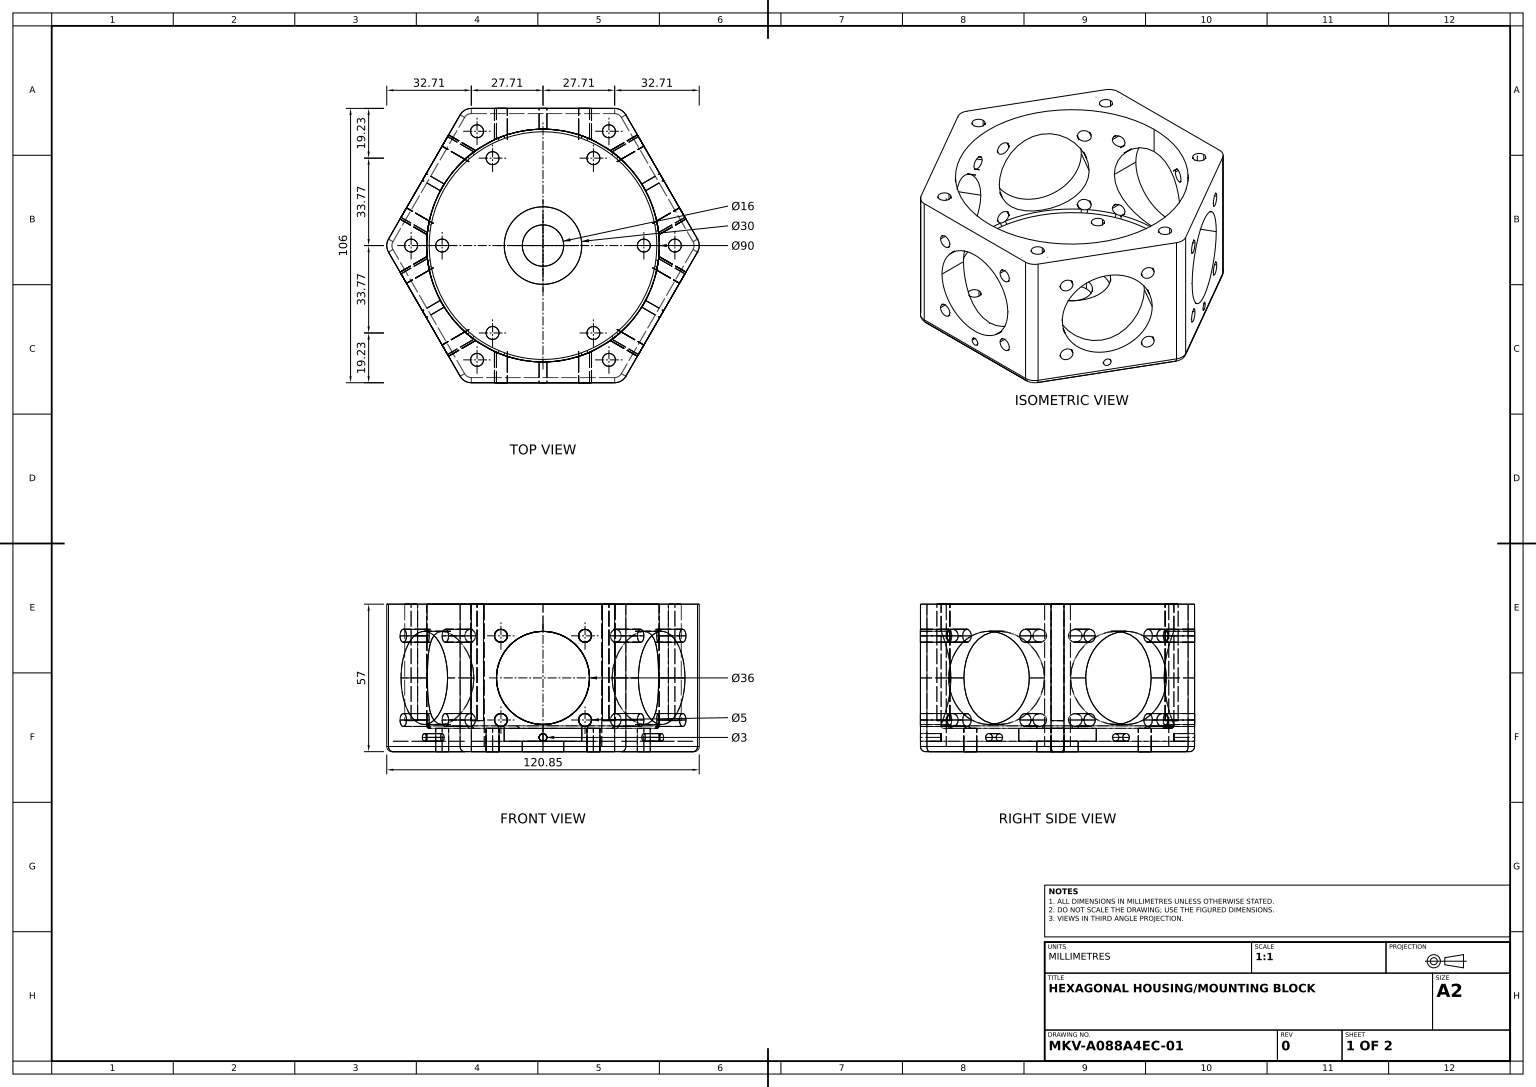
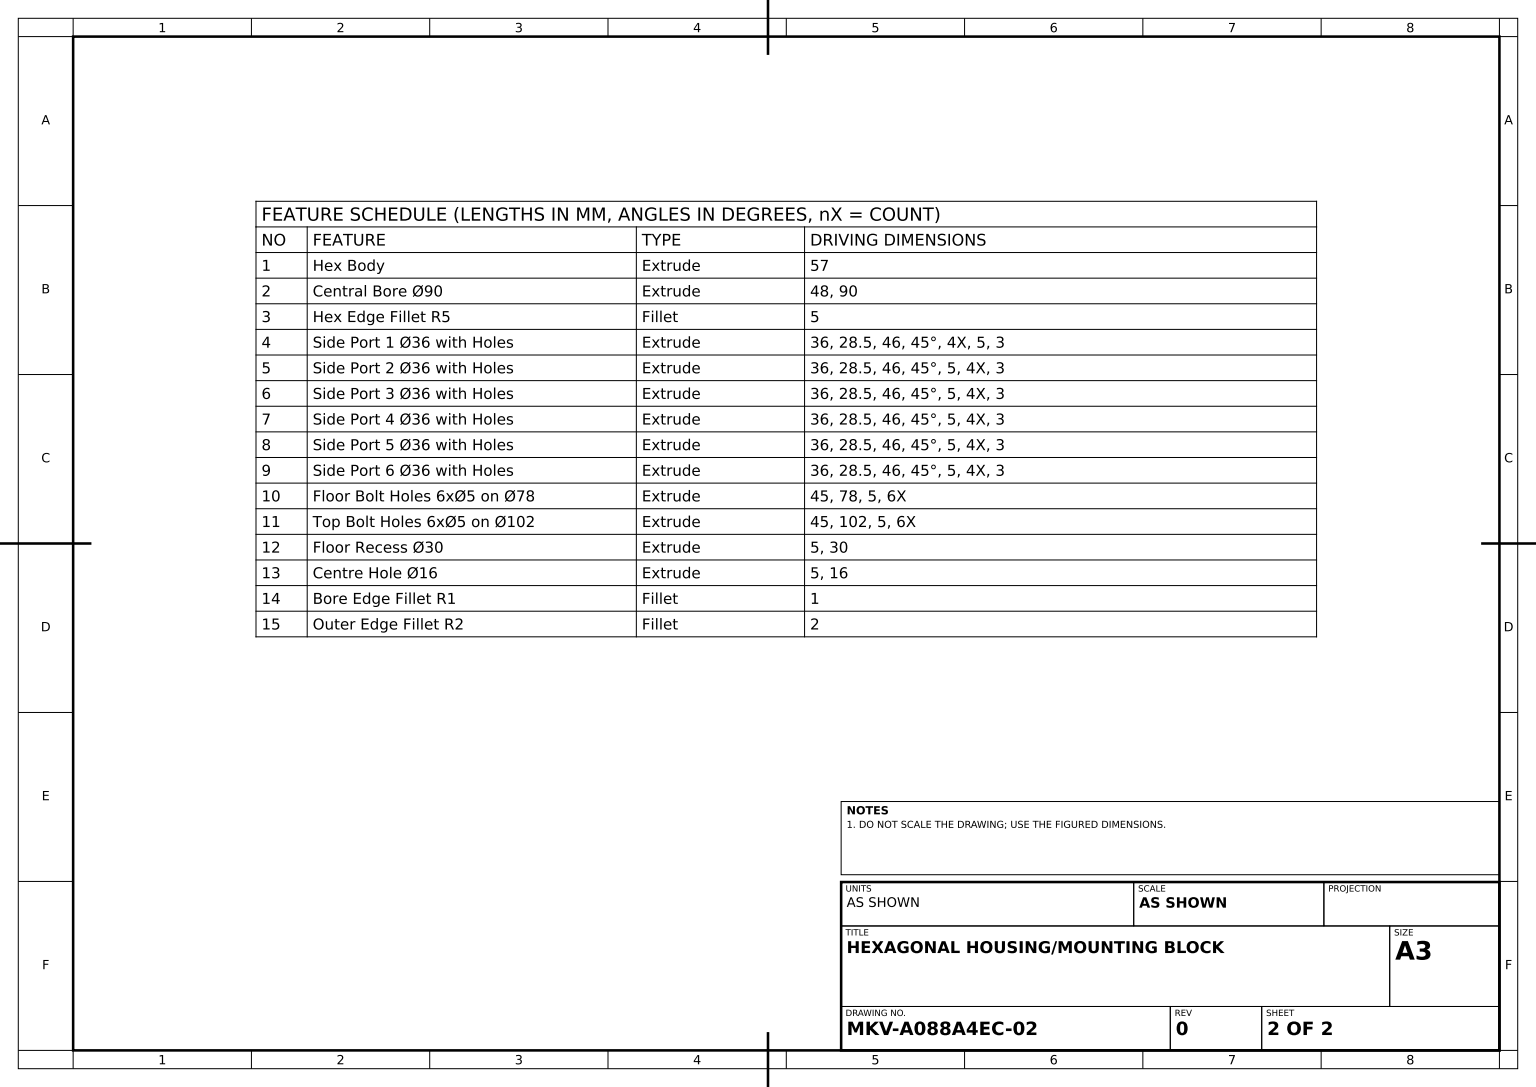
from build123d import *

# Parameters (mm, degrees)
HEX_BODY_DEPTH                       = 57
CENTRAL_BORE_SKETCH_R                = 45
CENTRAL_BORE_90_DEPTH                = 48
HEX_EDGE_FILLET_R5_R                 = 5
SIDE_PORT_1_36_WITH_HOLES_REACH      = 136.671
SIDE_PORT_1_36_WITH_HOLES_END_RADIUS = 45
SIDE_PORT_1_SKETCH_R                 = 18
SIDE_PORT_1_SKETCH_R_2               = 2.5
SIDE_PORT_1_SKETCH_R_3               = 1.5
SIDE_PORT_2_36_WITH_HOLES_REACH      = 146.479
SIDE_PORT_2_36_WITH_HOLES_END_RADIUS = 45
SIDE_PORT_2_SKETCH_R                 = 18
SIDE_PORT_2_SKETCH_R_2               = 2.5
SIDE_PORT_2_SKETCH_R_3               = 1.5
SIDE_PORT_3_36_WITH_HOLES_REACH      = 146.479
SIDE_PORT_3_36_WITH_HOLES_END_RADIUS = 45
SIDE_PORT_3_SKETCH_R                 = 18
SIDE_PORT_3_SKETCH_R_2               = 2.5
SIDE_PORT_3_SKETCH_R_3               = 1.5
SIDE_PORT_4_36_WITH_HOLES_REACH      = 136.671
SIDE_PORT_4_36_WITH_HOLES_END_RADIUS = 45
SIDE_PORT_4_SKETCH_R                 = 18
SIDE_PORT_4_SKETCH_R_2               = 2.5
SIDE_PORT_4_SKETCH_R_3               = 1.5
SIDE_PORT_5_36_WITH_HOLES_REACH      = 146.479
SIDE_PORT_5_36_WITH_HOLES_END_RADIUS = 45
SIDE_PORT_5_SKETCH_R                 = 18
SIDE_PORT_5_SKETCH_R_2               = 2.5
SIDE_PORT_5_SKETCH_R_3               = 1.5
SIDE_PORT_6_36_WITH_HOLES_REACH      = 146.479
SIDE_PORT_6_36_WITH_HOLES_END_RADIUS = 45
SIDE_PORT_6_SKETCH_R                 = 18
SIDE_PORT_6_SKETCH_R_2               = 2.5
SIDE_PORT_6_SKETCH_R_3               = 1.5
FLOOR_BOLT_CIRCLE_SKETCH_R           = 2.5
FLOOR_BOLT_HOLES_6X_5_ON_78_DEPTH    = 45
TOP_BOLT_CIRCLE_SKETCH_R             = 2.5
TOP_BOLT_HOLES_6X_5_ON_102_DEPTH     = 45
FLOOR_RECESS_SKETCH_R                = 15
FLOOR_RECESS_30_DEPTH                = 5
CENTRE_HOLE_SKETCH_R                 = 8
CENTRE_HOLE_16_DEPTH                 = 5
BORE_EDGE_FILLET_R1_R                = 1
OUTER_EDGE_FILLET_R2_R               = 2


with BuildPart() as part:
    # Hex Body Profile Sketch → Hex Body (new body)
    with BuildSketch(Plane(origin=(0, 0, 0), x_dir=(1, 0, 0), z_dir=(0, 1, 0))):
        Polygon((61.199128534, 0), (30.599564267, 53), (-30.599564267, 53), (-61.199128534, 0), (-30.599564267, -53), (30.599564267, -53), align=None)
    extrude(amount=HEX_BODY_DEPTH)

    # Central Bore Sketch → Central Bore Ø90 (cut)
    with BuildSketch(Plane(origin=(0, 57, 0), x_dir=(1, 0, 0), z_dir=(0, 1, 0))):
        with Locations(Location((0, 0, 0), (0, 0, 270))):
            Circle(CENTRAL_BORE_SKETCH_R)
    extrude(amount=-CENTRAL_BORE_90_DEPTH, mode=Mode.SUBTRACT)

    # Hex Edge Fillet R5
    hex_edge_fillet_r5_edges = [part.edges().sort_by_distance(p)[0] for p in [
        (30.599564267, 28.5, 53),
        (-30.599564267, 28.5, 53),
        (-61.199128534, 28.5, 0),
        (-30.599564267, 28.5, -53),
        (30.599564267, 28.5, -53),
        (61.199128534, 28.5, 0),
    ]]
    fillet(hex_edge_fillet_r5_edges, radius=HEX_EDGE_FILLET_R5_R)

    # Side Port 1 Ø36 with Holes: up to this cylinder (the profile starts outside it)
    side_port_1_36_with_holes_end = Plane(origin=(0, 25.131728, 0), z_dir=(0, 1, 0)) * Cylinder(SIDE_PORT_1_36_WITH_HOLES_END_RADIUS, 403.605456, mode=Mode.PRIVATE)
    # Side Port 1 Sketch → Side Port 1 Ø36 with Holes (cut, up to the surface)
    with BuildSketch(Plane(origin=(0, 0, -53), x_dir=(-1, 0, 0), z_dir=(0, 0, -1)), mode=Mode.PRIVATE) as side_port_1_36_with_holes_sk1:
        with Locations((0, 28.5)):
            Circle(SIDE_PORT_1_SKETCH_R)
    side_port_1_36_with_holes_tool1 = extrude(side_port_1_36_with_holes_sk1.sketch, amount=-SIDE_PORT_1_36_WITH_HOLES_REACH, mode=Mode.PRIVATE) - side_port_1_36_with_holes_end
    add(side_port_1_36_with_holes_tool1.solids().sort_by_distance((0, 28.5, -53))[0], mode=Mode.SUBTRACT)
    # Side Port 1 Sketch → Side Port 1 Ø36 with Holes (cut, up to the surface)
    with BuildSketch(Plane(origin=(0, 0, -53), x_dir=(-1, 0, 0), z_dir=(0, 0, -1)), mode=Mode.PRIVATE) as side_port_1_36_with_holes_sk2:
        with Locations((16.263455967, 44.763455967)):
            Circle(SIDE_PORT_1_SKETCH_R_2)
    side_port_1_36_with_holes_tool2 = extrude(side_port_1_36_with_holes_sk2.sketch, amount=-SIDE_PORT_1_36_WITH_HOLES_REACH, mode=Mode.PRIVATE) - side_port_1_36_with_holes_end
    add(side_port_1_36_with_holes_tool2.solids().sort_by_distance((-16.263456, 44.763456, -53))[0], mode=Mode.SUBTRACT)
    # Side Port 1 Sketch → Side Port 1 Ø36 with Holes (cut, up to the surface)
    with BuildSketch(Plane(origin=(0, 0, -53), x_dir=(-1, 0, 0), z_dir=(0, 0, -1)), mode=Mode.PRIVATE) as side_port_1_36_with_holes_sk3:
        with Locations((16.263455967, 12.236544033)):
            Circle(SIDE_PORT_1_SKETCH_R_2)
    side_port_1_36_with_holes_tool3 = extrude(side_port_1_36_with_holes_sk3.sketch, amount=-SIDE_PORT_1_36_WITH_HOLES_REACH, mode=Mode.PRIVATE) - side_port_1_36_with_holes_end
    add(side_port_1_36_with_holes_tool3.solids().sort_by_distance((-16.263456, 12.236544, -53))[0], mode=Mode.SUBTRACT)
    # Side Port 1 Sketch → Side Port 1 Ø36 with Holes (cut, up to the surface)
    with BuildSketch(Plane(origin=(0, 0, -53), x_dir=(-1, 0, 0), z_dir=(0, 0, -1)), mode=Mode.PRIVATE) as side_port_1_36_with_holes_sk4:
        with Locations((-16.263455967, 12.236544033)):
            Circle(SIDE_PORT_1_SKETCH_R_2)
    side_port_1_36_with_holes_tool4 = extrude(side_port_1_36_with_holes_sk4.sketch, amount=-SIDE_PORT_1_36_WITH_HOLES_REACH, mode=Mode.PRIVATE) - side_port_1_36_with_holes_end
    add(side_port_1_36_with_holes_tool4.solids().sort_by_distance((16.263456, 12.236544, -53))[0], mode=Mode.SUBTRACT)
    # Side Port 1 Sketch → Side Port 1 Ø36 with Holes (cut, up to the surface)
    with BuildSketch(Plane(origin=(0, 0, -53), x_dir=(-1, 0, 0), z_dir=(0, 0, -1)), mode=Mode.PRIVATE) as side_port_1_36_with_holes_sk5:
        with Locations((-16.263455967, 44.763455967)):
            Circle(SIDE_PORT_1_SKETCH_R_2)
    side_port_1_36_with_holes_tool5 = extrude(side_port_1_36_with_holes_sk5.sketch, amount=-SIDE_PORT_1_36_WITH_HOLES_REACH, mode=Mode.PRIVATE) - side_port_1_36_with_holes_end
    add(side_port_1_36_with_holes_tool5.solids().sort_by_distance((16.263456, 44.763456, -53))[0], mode=Mode.SUBTRACT)
    # Side Port 1 Sketch → Side Port 1 Ø36 with Holes (cut, up to the surface)
    with BuildSketch(Plane(origin=(0, 0, -53), x_dir=(-1, 0, 0), z_dir=(0, 0, -1)), mode=Mode.PRIVATE) as side_port_1_36_with_holes_sk6:
        with Locations((0, 5.5)):
            Circle(SIDE_PORT_1_SKETCH_R_3)
    side_port_1_36_with_holes_tool6 = extrude(side_port_1_36_with_holes_sk6.sketch, amount=-SIDE_PORT_1_36_WITH_HOLES_REACH, mode=Mode.PRIVATE) - side_port_1_36_with_holes_end
    add(side_port_1_36_with_holes_tool6.solids().sort_by_distance((0, 5.5, -53))[0], mode=Mode.SUBTRACT)

    # Side Port 2 Ø36 with Holes: up to this cylinder (the profile starts outside it)
    side_port_2_36_with_holes_end = Plane(origin=(0, 25.131728, 0), z_dir=(0, 1, 0)) * Cylinder(SIDE_PORT_2_36_WITH_HOLES_END_RADIUS, 423.221456, mode=Mode.PRIVATE)
    # Side Port 2 Sketch → Side Port 2 Ø36 with Holes (cut, up to the surface)
    with BuildSketch(Plane(origin=(-45.899346401, 0, -26.5), x_dir=(-0.49999999999999484, 0, 0.8660254037844416), z_dir=(-0.8660254037844416, 0, -0.49999999999999484)), mode=Mode.PRIVATE) as side_port_2_36_with_holes_sk1:
        with Locations((0, 28.5)):
            Circle(SIDE_PORT_2_SKETCH_R)
    side_port_2_36_with_holes_tool1 = extrude(side_port_2_36_with_holes_sk1.sketch, amount=-SIDE_PORT_2_36_WITH_HOLES_REACH, mode=Mode.PRIVATE) - side_port_2_36_with_holes_end
    add(side_port_2_36_with_holes_tool1.solids().sort_by_distance((-45.899346, 28.5, -26.5))[0], mode=Mode.SUBTRACT)
    # Side Port 2 Sketch → Side Port 2 Ø36 with Holes (cut, up to the surface)
    with BuildSketch(Plane(origin=(-45.899346401, 0, -26.5), x_dir=(-0.49999999999999484, 0, 0.8660254037844416), z_dir=(-0.8660254037844416, 0, -0.49999999999999484)), mode=Mode.PRIVATE) as side_port_2_36_with_holes_sk2:
        with Locations((16.263455967, 44.763455967)):
            Circle(SIDE_PORT_2_SKETCH_R_2)
    side_port_2_36_with_holes_tool2 = extrude(side_port_2_36_with_holes_sk2.sketch, amount=-SIDE_PORT_2_36_WITH_HOLES_REACH, mode=Mode.PRIVATE) - side_port_2_36_with_holes_end
    add(side_port_2_36_with_holes_tool2.solids().sort_by_distance((-54.031074, 44.763456, -12.415434))[0], mode=Mode.SUBTRACT)
    # Side Port 2 Sketch → Side Port 2 Ø36 with Holes (cut, up to the surface)
    with BuildSketch(Plane(origin=(-45.899346401, 0, -26.5), x_dir=(-0.49999999999999484, 0, 0.8660254037844416), z_dir=(-0.8660254037844416, 0, -0.49999999999999484)), mode=Mode.PRIVATE) as side_port_2_36_with_holes_sk3:
        with Locations((16.263455967, 12.236544033)):
            Circle(SIDE_PORT_2_SKETCH_R_2)
    side_port_2_36_with_holes_tool3 = extrude(side_port_2_36_with_holes_sk3.sketch, amount=-SIDE_PORT_2_36_WITH_HOLES_REACH, mode=Mode.PRIVATE) - side_port_2_36_with_holes_end
    add(side_port_2_36_with_holes_tool3.solids().sort_by_distance((-54.031074, 12.236544, -12.415434))[0], mode=Mode.SUBTRACT)
    # Side Port 2 Sketch → Side Port 2 Ø36 with Holes (cut, up to the surface)
    with BuildSketch(Plane(origin=(-45.899346401, 0, -26.5), x_dir=(-0.49999999999999484, 0, 0.8660254037844416), z_dir=(-0.8660254037844416, 0, -0.49999999999999484)), mode=Mode.PRIVATE) as side_port_2_36_with_holes_sk4:
        with Locations((-16.263455967, 12.236544033)):
            Circle(SIDE_PORT_2_SKETCH_R_2)
    side_port_2_36_with_holes_tool4 = extrude(side_port_2_36_with_holes_sk4.sketch, amount=-SIDE_PORT_2_36_WITH_HOLES_REACH, mode=Mode.PRIVATE) - side_port_2_36_with_holes_end
    add(side_port_2_36_with_holes_tool4.solids().sort_by_distance((-37.767618, 12.236544, -40.584566))[0], mode=Mode.SUBTRACT)
    # Side Port 2 Sketch → Side Port 2 Ø36 with Holes (cut, up to the surface)
    with BuildSketch(Plane(origin=(-45.899346401, 0, -26.5), x_dir=(-0.49999999999999484, 0, 0.8660254037844416), z_dir=(-0.8660254037844416, 0, -0.49999999999999484)), mode=Mode.PRIVATE) as side_port_2_36_with_holes_sk5:
        with Locations((-16.263455967, 44.763455967)):
            Circle(SIDE_PORT_2_SKETCH_R_2)
    side_port_2_36_with_holes_tool5 = extrude(side_port_2_36_with_holes_sk5.sketch, amount=-SIDE_PORT_2_36_WITH_HOLES_REACH, mode=Mode.PRIVATE) - side_port_2_36_with_holes_end
    add(side_port_2_36_with_holes_tool5.solids().sort_by_distance((-37.767618, 44.763456, -40.584566))[0], mode=Mode.SUBTRACT)
    # Side Port 2 Sketch → Side Port 2 Ø36 with Holes (cut, up to the surface)
    with BuildSketch(Plane(origin=(-45.899346401, 0, -26.5), x_dir=(-0.49999999999999484, 0, 0.8660254037844416), z_dir=(-0.8660254037844416, 0, -0.49999999999999484)), mode=Mode.PRIVATE) as side_port_2_36_with_holes_sk6:
        with Locations((0, 5.5)):
            Circle(SIDE_PORT_2_SKETCH_R_3)
    side_port_2_36_with_holes_tool6 = extrude(side_port_2_36_with_holes_sk6.sketch, amount=-SIDE_PORT_2_36_WITH_HOLES_REACH, mode=Mode.PRIVATE) - side_port_2_36_with_holes_end
    add(side_port_2_36_with_holes_tool6.solids().sort_by_distance((-45.899346, 5.5, -26.5))[0], mode=Mode.SUBTRACT)

    # Side Port 3 Ø36 with Holes: up to this cylinder (the profile starts outside it)
    side_port_3_36_with_holes_end = Plane(origin=(0, 25.131728, 0), z_dir=(0, 1, 0)) * Cylinder(SIDE_PORT_3_36_WITH_HOLES_END_RADIUS, 423.221456, mode=Mode.PRIVATE)
    # Side Port 3 Sketch → Side Port 3 Ø36 with Holes (cut, up to the surface)
    with BuildSketch(Plane(origin=(-45.899346401, 0, 26.5), x_dir=(0.5000000000000071, 0, 0.8660254037844346), z_dir=(-0.8660254037844345, 0, 0.500000000000007)), mode=Mode.PRIVATE) as side_port_3_36_with_holes_sk1:
        with Locations((0, 28.5)):
            Circle(SIDE_PORT_3_SKETCH_R)
    side_port_3_36_with_holes_tool1 = extrude(side_port_3_36_with_holes_sk1.sketch, amount=-SIDE_PORT_3_36_WITH_HOLES_REACH, mode=Mode.PRIVATE) - side_port_3_36_with_holes_end
    add(side_port_3_36_with_holes_tool1.solids().sort_by_distance((-45.899346, 28.5, 26.5))[0], mode=Mode.SUBTRACT)
    # Side Port 3 Sketch → Side Port 3 Ø36 with Holes (cut, up to the surface)
    with BuildSketch(Plane(origin=(-45.899346401, 0, 26.5), x_dir=(0.5000000000000071, 0, 0.8660254037844346), z_dir=(-0.8660254037844345, 0, 0.500000000000007)), mode=Mode.PRIVATE) as side_port_3_36_with_holes_sk2:
        with Locations((16.263455967, 44.763455967)):
            Circle(SIDE_PORT_3_SKETCH_R_2)
    side_port_3_36_with_holes_tool2 = extrude(side_port_3_36_with_holes_sk2.sketch, amount=-SIDE_PORT_3_36_WITH_HOLES_REACH, mode=Mode.PRIVATE) - side_port_3_36_with_holes_end
    add(side_port_3_36_with_holes_tool2.solids().sort_by_distance((-37.767618, 44.763456, 40.584566))[0], mode=Mode.SUBTRACT)
    # Side Port 3 Sketch → Side Port 3 Ø36 with Holes (cut, up to the surface)
    with BuildSketch(Plane(origin=(-45.899346401, 0, 26.5), x_dir=(0.5000000000000071, 0, 0.8660254037844346), z_dir=(-0.8660254037844345, 0, 0.500000000000007)), mode=Mode.PRIVATE) as side_port_3_36_with_holes_sk3:
        with Locations((16.263455967, 12.236544033)):
            Circle(SIDE_PORT_3_SKETCH_R_2)
    side_port_3_36_with_holes_tool3 = extrude(side_port_3_36_with_holes_sk3.sketch, amount=-SIDE_PORT_3_36_WITH_HOLES_REACH, mode=Mode.PRIVATE) - side_port_3_36_with_holes_end
    add(side_port_3_36_with_holes_tool3.solids().sort_by_distance((-37.767618, 12.236544, 40.584566))[0], mode=Mode.SUBTRACT)
    # Side Port 3 Sketch → Side Port 3 Ø36 with Holes (cut, up to the surface)
    with BuildSketch(Plane(origin=(-45.899346401, 0, 26.5), x_dir=(0.5000000000000071, 0, 0.8660254037844346), z_dir=(-0.8660254037844345, 0, 0.500000000000007)), mode=Mode.PRIVATE) as side_port_3_36_with_holes_sk4:
        with Locations((-16.263455967, 12.236544033)):
            Circle(SIDE_PORT_3_SKETCH_R_2)
    side_port_3_36_with_holes_tool4 = extrude(side_port_3_36_with_holes_sk4.sketch, amount=-SIDE_PORT_3_36_WITH_HOLES_REACH, mode=Mode.PRIVATE) - side_port_3_36_with_holes_end
    add(side_port_3_36_with_holes_tool4.solids().sort_by_distance((-54.031074, 12.236544, 12.415434))[0], mode=Mode.SUBTRACT)
    # Side Port 3 Sketch → Side Port 3 Ø36 with Holes (cut, up to the surface)
    with BuildSketch(Plane(origin=(-45.899346401, 0, 26.5), x_dir=(0.5000000000000071, 0, 0.8660254037844346), z_dir=(-0.8660254037844345, 0, 0.500000000000007)), mode=Mode.PRIVATE) as side_port_3_36_with_holes_sk5:
        with Locations((-16.263455967, 44.763455967)):
            Circle(SIDE_PORT_3_SKETCH_R_2)
    side_port_3_36_with_holes_tool5 = extrude(side_port_3_36_with_holes_sk5.sketch, amount=-SIDE_PORT_3_36_WITH_HOLES_REACH, mode=Mode.PRIVATE) - side_port_3_36_with_holes_end
    add(side_port_3_36_with_holes_tool5.solids().sort_by_distance((-54.031074, 44.763456, 12.415434))[0], mode=Mode.SUBTRACT)
    # Side Port 3 Sketch → Side Port 3 Ø36 with Holes (cut, up to the surface)
    with BuildSketch(Plane(origin=(-45.899346401, 0, 26.5), x_dir=(0.5000000000000071, 0, 0.8660254037844346), z_dir=(-0.8660254037844345, 0, 0.500000000000007)), mode=Mode.PRIVATE) as side_port_3_36_with_holes_sk6:
        with Locations((0, 5.5)):
            Circle(SIDE_PORT_3_SKETCH_R_3)
    side_port_3_36_with_holes_tool6 = extrude(side_port_3_36_with_holes_sk6.sketch, amount=-SIDE_PORT_3_36_WITH_HOLES_REACH, mode=Mode.PRIVATE) - side_port_3_36_with_holes_end
    add(side_port_3_36_with_holes_tool6.solids().sort_by_distance((-45.899346, 5.5, 26.5))[0], mode=Mode.SUBTRACT)

    # Side Port 4 Ø36 with Holes: up to this cylinder (the profile starts outside it)
    side_port_4_36_with_holes_end = Plane(origin=(0, 25.131728, 0), z_dir=(0, 1, 0)) * Cylinder(SIDE_PORT_4_36_WITH_HOLES_END_RADIUS, 403.605456, mode=Mode.PRIVATE)
    # Side Port 4 Sketch → Side Port 4 Ø36 with Holes (cut, up to the surface)
    with BuildSketch(Plane.XY.offset(53), mode=Mode.PRIVATE) as side_port_4_36_with_holes_sk1:
        with Locations(Location((0, 28.5, 0), (0, 0, 180))):
            Circle(SIDE_PORT_4_SKETCH_R)
    side_port_4_36_with_holes_tool1 = extrude(side_port_4_36_with_holes_sk1.sketch, amount=-SIDE_PORT_4_36_WITH_HOLES_REACH, mode=Mode.PRIVATE) - side_port_4_36_with_holes_end
    add(side_port_4_36_with_holes_tool1.solids().sort_by_distance((0, 28.5, 53))[0], mode=Mode.SUBTRACT)
    # Side Port 4 Sketch → Side Port 4 Ø36 with Holes (cut, up to the surface)
    with BuildSketch(Plane.XY.offset(53), mode=Mode.PRIVATE) as side_port_4_36_with_holes_sk2:
        with Locations(Location((16.263455967, 44.763455967, 0), (0, 0, 180))):
            Circle(SIDE_PORT_4_SKETCH_R_2)
    side_port_4_36_with_holes_tool2 = extrude(side_port_4_36_with_holes_sk2.sketch, amount=-SIDE_PORT_4_36_WITH_HOLES_REACH, mode=Mode.PRIVATE) - side_port_4_36_with_holes_end
    add(side_port_4_36_with_holes_tool2.solids().sort_by_distance((16.263456, 44.763456, 53))[0], mode=Mode.SUBTRACT)
    # Side Port 4 Sketch → Side Port 4 Ø36 with Holes (cut, up to the surface)
    with BuildSketch(Plane.XY.offset(53), mode=Mode.PRIVATE) as side_port_4_36_with_holes_sk3:
        with Locations(Location((16.263455967, 12.236544033, 0), (0, 0, 180))):
            Circle(SIDE_PORT_4_SKETCH_R_2)
    side_port_4_36_with_holes_tool3 = extrude(side_port_4_36_with_holes_sk3.sketch, amount=-SIDE_PORT_4_36_WITH_HOLES_REACH, mode=Mode.PRIVATE) - side_port_4_36_with_holes_end
    add(side_port_4_36_with_holes_tool3.solids().sort_by_distance((16.263456, 12.236544, 53))[0], mode=Mode.SUBTRACT)
    # Side Port 4 Sketch → Side Port 4 Ø36 with Holes (cut, up to the surface)
    with BuildSketch(Plane.XY.offset(53), mode=Mode.PRIVATE) as side_port_4_36_with_holes_sk4:
        with Locations(Location((-16.263455967, 12.236544033, 0), (0, 0, 180))):
            Circle(SIDE_PORT_4_SKETCH_R_2)
    side_port_4_36_with_holes_tool4 = extrude(side_port_4_36_with_holes_sk4.sketch, amount=-SIDE_PORT_4_36_WITH_HOLES_REACH, mode=Mode.PRIVATE) - side_port_4_36_with_holes_end
    add(side_port_4_36_with_holes_tool4.solids().sort_by_distance((-16.263456, 12.236544, 53))[0], mode=Mode.SUBTRACT)
    # Side Port 4 Sketch → Side Port 4 Ø36 with Holes (cut, up to the surface)
    with BuildSketch(Plane.XY.offset(53), mode=Mode.PRIVATE) as side_port_4_36_with_holes_sk5:
        with Locations(Location((-16.263455967, 44.763455967, 0), (0, 0, 180))):
            Circle(SIDE_PORT_4_SKETCH_R_2)
    side_port_4_36_with_holes_tool5 = extrude(side_port_4_36_with_holes_sk5.sketch, amount=-SIDE_PORT_4_36_WITH_HOLES_REACH, mode=Mode.PRIVATE) - side_port_4_36_with_holes_end
    add(side_port_4_36_with_holes_tool5.solids().sort_by_distance((-16.263456, 44.763456, 53))[0], mode=Mode.SUBTRACT)
    # Side Port 4 Sketch → Side Port 4 Ø36 with Holes (cut, up to the surface)
    with BuildSketch(Plane.XY.offset(53), mode=Mode.PRIVATE) as side_port_4_36_with_holes_sk6:
        with Locations(Location((0, 5.5, 0), (0, 0, 180))):
            Circle(SIDE_PORT_4_SKETCH_R_3)
    side_port_4_36_with_holes_tool6 = extrude(side_port_4_36_with_holes_sk6.sketch, amount=-SIDE_PORT_4_36_WITH_HOLES_REACH, mode=Mode.PRIVATE) - side_port_4_36_with_holes_end
    add(side_port_4_36_with_holes_tool6.solids().sort_by_distance((0, 5.5, 53))[0], mode=Mode.SUBTRACT)

    # Side Port 5 Ø36 with Holes: up to this cylinder (the profile starts outside it)
    side_port_5_36_with_holes_end = Plane(origin=(0, 25.131728, 0), z_dir=(0, 1, 0)) * Cylinder(SIDE_PORT_5_36_WITH_HOLES_END_RADIUS, 423.221456, mode=Mode.PRIVATE)
    # Side Port 5 Sketch → Side Port 5 Ø36 with Holes (cut, up to the surface)
    with BuildSketch(Plane(origin=(45.899346401, 0, 26.5), x_dir=(0.49999999999999484, 0, -0.8660254037844417), z_dir=(0.8660254037844417, 0, 0.49999999999999484)), mode=Mode.PRIVATE) as side_port_5_36_with_holes_sk1:
        with Locations(Location((0, 28.5, 0), (0, 0, 180))):
            Circle(SIDE_PORT_5_SKETCH_R)
    side_port_5_36_with_holes_tool1 = extrude(side_port_5_36_with_holes_sk1.sketch, amount=-SIDE_PORT_5_36_WITH_HOLES_REACH, mode=Mode.PRIVATE) - side_port_5_36_with_holes_end
    add(side_port_5_36_with_holes_tool1.solids().sort_by_distance((45.899346, 28.5, 26.5))[0], mode=Mode.SUBTRACT)
    # Side Port 5 Sketch → Side Port 5 Ø36 with Holes (cut, up to the surface)
    with BuildSketch(Plane(origin=(45.899346401, 0, 26.5), x_dir=(0.49999999999999484, 0, -0.8660254037844417), z_dir=(0.8660254037844417, 0, 0.49999999999999484)), mode=Mode.PRIVATE) as side_port_5_36_with_holes_sk2:
        with Locations(Location((16.263455967, 44.763455967, 0), (0, 0, 180))):
            Circle(SIDE_PORT_5_SKETCH_R_2)
    side_port_5_36_with_holes_tool2 = extrude(side_port_5_36_with_holes_sk2.sketch, amount=-SIDE_PORT_5_36_WITH_HOLES_REACH, mode=Mode.PRIVATE) - side_port_5_36_with_holes_end
    add(side_port_5_36_with_holes_tool2.solids().sort_by_distance((54.031074, 44.763456, 12.415434))[0], mode=Mode.SUBTRACT)
    # Side Port 5 Sketch → Side Port 5 Ø36 with Holes (cut, up to the surface)
    with BuildSketch(Plane(origin=(45.899346401, 0, 26.5), x_dir=(0.49999999999999484, 0, -0.8660254037844417), z_dir=(0.8660254037844417, 0, 0.49999999999999484)), mode=Mode.PRIVATE) as side_port_5_36_with_holes_sk3:
        with Locations(Location((16.263455967, 12.236544033, 0), (0, 0, 180))):
            Circle(SIDE_PORT_5_SKETCH_R_2)
    side_port_5_36_with_holes_tool3 = extrude(side_port_5_36_with_holes_sk3.sketch, amount=-SIDE_PORT_5_36_WITH_HOLES_REACH, mode=Mode.PRIVATE) - side_port_5_36_with_holes_end
    add(side_port_5_36_with_holes_tool3.solids().sort_by_distance((54.031074, 12.236544, 12.415434))[0], mode=Mode.SUBTRACT)
    # Side Port 5 Sketch → Side Port 5 Ø36 with Holes (cut, up to the surface)
    with BuildSketch(Plane(origin=(45.899346401, 0, 26.5), x_dir=(0.49999999999999484, 0, -0.8660254037844417), z_dir=(0.8660254037844417, 0, 0.49999999999999484)), mode=Mode.PRIVATE) as side_port_5_36_with_holes_sk4:
        with Locations(Location((-16.263455967, 12.236544033, 0), (0, 0, 180))):
            Circle(SIDE_PORT_5_SKETCH_R_2)
    side_port_5_36_with_holes_tool4 = extrude(side_port_5_36_with_holes_sk4.sketch, amount=-SIDE_PORT_5_36_WITH_HOLES_REACH, mode=Mode.PRIVATE) - side_port_5_36_with_holes_end
    add(side_port_5_36_with_holes_tool4.solids().sort_by_distance((37.767618, 12.236544, 40.584566))[0], mode=Mode.SUBTRACT)
    # Side Port 5 Sketch → Side Port 5 Ø36 with Holes (cut, up to the surface)
    with BuildSketch(Plane(origin=(45.899346401, 0, 26.5), x_dir=(0.49999999999999484, 0, -0.8660254037844417), z_dir=(0.8660254037844417, 0, 0.49999999999999484)), mode=Mode.PRIVATE) as side_port_5_36_with_holes_sk5:
        with Locations(Location((-16.263455967, 44.763455967, 0), (0, 0, 180))):
            Circle(SIDE_PORT_5_SKETCH_R_2)
    side_port_5_36_with_holes_tool5 = extrude(side_port_5_36_with_holes_sk5.sketch, amount=-SIDE_PORT_5_36_WITH_HOLES_REACH, mode=Mode.PRIVATE) - side_port_5_36_with_holes_end
    add(side_port_5_36_with_holes_tool5.solids().sort_by_distance((37.767618, 44.763456, 40.584566))[0], mode=Mode.SUBTRACT)
    # Side Port 5 Sketch → Side Port 5 Ø36 with Holes (cut, up to the surface)
    with BuildSketch(Plane(origin=(45.899346401, 0, 26.5), x_dir=(0.49999999999999484, 0, -0.8660254037844417), z_dir=(0.8660254037844417, 0, 0.49999999999999484)), mode=Mode.PRIVATE) as side_port_5_36_with_holes_sk6:
        with Locations(Location((0, 5.5, 0), (0, 0, 180))):
            Circle(SIDE_PORT_5_SKETCH_R_3)
    side_port_5_36_with_holes_tool6 = extrude(side_port_5_36_with_holes_sk6.sketch, amount=-SIDE_PORT_5_36_WITH_HOLES_REACH, mode=Mode.PRIVATE) - side_port_5_36_with_holes_end
    add(side_port_5_36_with_holes_tool6.solids().sort_by_distance((45.899346, 5.5, 26.5))[0], mode=Mode.SUBTRACT)

    # Side Port 6 Ø36 with Holes: up to this cylinder (the profile starts outside it)
    side_port_6_36_with_holes_end = Plane(origin=(0, 25.131728, 0), z_dir=(0, 1, 0)) * Cylinder(SIDE_PORT_6_36_WITH_HOLES_END_RADIUS, 423.221456, mode=Mode.PRIVATE)
    # Side Port 6 Sketch → Side Port 6 Ø36 with Holes (cut, up to the surface)
    with BuildSketch(Plane(origin=(45.899346401, 0, -26.5), x_dir=(-0.5000000000000011, 0, -0.866025403784438), z_dir=(0.8660254037844382, 0, -0.5000000000000011)), mode=Mode.PRIVATE) as side_port_6_36_with_holes_sk1:
        with Locations(Location((0, 28.5, 0), (0, 0, 180))):
            Circle(SIDE_PORT_6_SKETCH_R)
    side_port_6_36_with_holes_tool1 = extrude(side_port_6_36_with_holes_sk1.sketch, amount=-SIDE_PORT_6_36_WITH_HOLES_REACH, mode=Mode.PRIVATE) - side_port_6_36_with_holes_end
    add(side_port_6_36_with_holes_tool1.solids().sort_by_distance((45.899346, 28.5, -26.5))[0], mode=Mode.SUBTRACT)
    # Side Port 6 Sketch → Side Port 6 Ø36 with Holes (cut, up to the surface)
    with BuildSketch(Plane(origin=(45.899346401, 0, -26.5), x_dir=(-0.5000000000000011, 0, -0.866025403784438), z_dir=(0.8660254037844382, 0, -0.5000000000000011)), mode=Mode.PRIVATE) as side_port_6_36_with_holes_sk2:
        with Locations(Location((16.263455967, 44.763455967, 0), (0, 0, 180))):
            Circle(SIDE_PORT_6_SKETCH_R_2)
    side_port_6_36_with_holes_tool2 = extrude(side_port_6_36_with_holes_sk2.sketch, amount=-SIDE_PORT_6_36_WITH_HOLES_REACH, mode=Mode.PRIVATE) - side_port_6_36_with_holes_end
    add(side_port_6_36_with_holes_tool2.solids().sort_by_distance((37.767618, 44.763456, -40.584566))[0], mode=Mode.SUBTRACT)
    # Side Port 6 Sketch → Side Port 6 Ø36 with Holes (cut, up to the surface)
    with BuildSketch(Plane(origin=(45.899346401, 0, -26.5), x_dir=(-0.5000000000000011, 0, -0.866025403784438), z_dir=(0.8660254037844382, 0, -0.5000000000000011)), mode=Mode.PRIVATE) as side_port_6_36_with_holes_sk3:
        with Locations(Location((16.263455967, 12.236544033, 0), (0, 0, 180))):
            Circle(SIDE_PORT_6_SKETCH_R_2)
    side_port_6_36_with_holes_tool3 = extrude(side_port_6_36_with_holes_sk3.sketch, amount=-SIDE_PORT_6_36_WITH_HOLES_REACH, mode=Mode.PRIVATE) - side_port_6_36_with_holes_end
    add(side_port_6_36_with_holes_tool3.solids().sort_by_distance((37.767618, 12.236544, -40.584566))[0], mode=Mode.SUBTRACT)
    # Side Port 6 Sketch → Side Port 6 Ø36 with Holes (cut, up to the surface)
    with BuildSketch(Plane(origin=(45.899346401, 0, -26.5), x_dir=(-0.5000000000000011, 0, -0.866025403784438), z_dir=(0.8660254037844382, 0, -0.5000000000000011)), mode=Mode.PRIVATE) as side_port_6_36_with_holes_sk4:
        with Locations(Location((-16.263455967, 12.236544033, 0), (0, 0, 180))):
            Circle(SIDE_PORT_6_SKETCH_R_2)
    side_port_6_36_with_holes_tool4 = extrude(side_port_6_36_with_holes_sk4.sketch, amount=-SIDE_PORT_6_36_WITH_HOLES_REACH, mode=Mode.PRIVATE) - side_port_6_36_with_holes_end
    add(side_port_6_36_with_holes_tool4.solids().sort_by_distance((54.031074, 12.236544, -12.415434))[0], mode=Mode.SUBTRACT)
    # Side Port 6 Sketch → Side Port 6 Ø36 with Holes (cut, up to the surface)
    with BuildSketch(Plane(origin=(45.899346401, 0, -26.5), x_dir=(-0.5000000000000011, 0, -0.866025403784438), z_dir=(0.8660254037844382, 0, -0.5000000000000011)), mode=Mode.PRIVATE) as side_port_6_36_with_holes_sk5:
        with Locations(Location((-16.263455967, 44.763455967, 0), (0, 0, 180))):
            Circle(SIDE_PORT_6_SKETCH_R_2)
    side_port_6_36_with_holes_tool5 = extrude(side_port_6_36_with_holes_sk5.sketch, amount=-SIDE_PORT_6_36_WITH_HOLES_REACH, mode=Mode.PRIVATE) - side_port_6_36_with_holes_end
    add(side_port_6_36_with_holes_tool5.solids().sort_by_distance((54.031074, 44.763456, -12.415434))[0], mode=Mode.SUBTRACT)
    # Side Port 6 Sketch → Side Port 6 Ø36 with Holes (cut, up to the surface)
    with BuildSketch(Plane(origin=(45.899346401, 0, -26.5), x_dir=(-0.5000000000000011, 0, -0.866025403784438), z_dir=(0.8660254037844382, 0, -0.5000000000000011)), mode=Mode.PRIVATE) as side_port_6_36_with_holes_sk6:
        with Locations(Location((0, 5.5, 0), (0, 0, 180))):
            Circle(SIDE_PORT_6_SKETCH_R_3)
    side_port_6_36_with_holes_tool6 = extrude(side_port_6_36_with_holes_sk6.sketch, amount=-SIDE_PORT_6_36_WITH_HOLES_REACH, mode=Mode.PRIVATE) - side_port_6_36_with_holes_end
    add(side_port_6_36_with_holes_tool6.solids().sort_by_distance((45.899346, 5.5, -26.5))[0], mode=Mode.SUBTRACT)

    # Floor Bolt Circle Sketch → Floor Bolt Holes 6xØ5 on Ø78 (cut)
    with BuildSketch(Plane(origin=(0, 9, 0), x_dir=(1, 0, 0), z_dir=(0, 1, 0))):
        with Locations(Location((39, 0, 0), (0, 0, 270))):
            Circle(FLOOR_BOLT_CIRCLE_SKETCH_R)
        with Locations(Location((19.5, -33.774990748, 0), (0, 0, 270))):
            Circle(FLOOR_BOLT_CIRCLE_SKETCH_R)
        with Locations(Location((-19.5, -33.774990748, 0), (0, 0, 270))):
            Circle(FLOOR_BOLT_CIRCLE_SKETCH_R)
        with Locations(Location((-39, 0, 0), (0, 0, 270))):
            Circle(FLOOR_BOLT_CIRCLE_SKETCH_R)
        with Locations(Location((-19.5, 33.774990748, 0), (0, 0, 270))):
            Circle(FLOOR_BOLT_CIRCLE_SKETCH_R)
        with Locations(Location((19.5, 33.774990748, 0), (0, 0, 270))):
            Circle(FLOOR_BOLT_CIRCLE_SKETCH_R)
    extrude(amount=-FLOOR_BOLT_HOLES_6X_5_ON_78_DEPTH, mode=Mode.SUBTRACT)

    # Top Bolt Circle Sketch → Top Bolt Holes 6xØ5 on Ø102 (cut)
    with BuildSketch(Plane(origin=(0, 57, 0), x_dir=(1, 0, 0), z_dir=(0, 1, 0))):
        with Locations(Location((51, 0, 0), (0, 0, 270))):
            Circle(TOP_BOLT_CIRCLE_SKETCH_R)
        with Locations(Location((25.5, -44.167295593, 0), (0, 0, 270))):
            Circle(TOP_BOLT_CIRCLE_SKETCH_R)
        with Locations(Location((-25.5, -44.167295593, 0), (0, 0, 270))):
            Circle(TOP_BOLT_CIRCLE_SKETCH_R)
        with Locations(Location((-51, 0, 0), (0, 0, 270))):
            Circle(TOP_BOLT_CIRCLE_SKETCH_R)
        with Locations(Location((-25.5, 44.167295593, 0), (0, 0, 270))):
            Circle(TOP_BOLT_CIRCLE_SKETCH_R)
        with Locations(Location((25.5, 44.167295593, 0), (0, 0, 270))):
            Circle(TOP_BOLT_CIRCLE_SKETCH_R)
    extrude(amount=-TOP_BOLT_HOLES_6X_5_ON_102_DEPTH, mode=Mode.SUBTRACT)

    # Floor Recess Sketch → Floor Recess Ø30 (cut)
    with BuildSketch(Plane(origin=(0, 9, 0), x_dir=(1, 0, 0), z_dir=(0, 1, 0))):
        with Locations(Location((0, 0, 0), (0, 0, 270))):
            Circle(FLOOR_RECESS_SKETCH_R)
    extrude(amount=-FLOOR_RECESS_30_DEPTH, mode=Mode.SUBTRACT)

    # Centre Hole Sketch → Centre Hole Ø16 (cut)
    with BuildSketch(Plane(origin=(0, 4, 0), x_dir=(1, 0, 0), z_dir=(0, 1, 0))):
        with Locations(Location((0, 0, 0), (0, 0, 270))):
            Circle(CENTRE_HOLE_SKETCH_R)
    extrude(amount=-CENTRE_HOLE_16_DEPTH, mode=Mode.SUBTRACT)

    # Bore Edge Fillet R1
    bore_edge_fillet_r1_edges = [part.edges().sort_by_distance(p)[0] for p in [
        (0, 9, -45),
    ]]
    fillet(bore_edge_fillet_r1_edges, radius=BORE_EDGE_FILLET_R1_R)

    # Outer Edge Fillet R2
    outer_edge_fillet_r2_edges = [part.edges().sort_by_distance(p)[0] for p in [
        (0, 0, -53),
        (45.899346401, 0, 26.5),
        (0, 0, 53),
        (-45.899346401, 0, 26.5),
        (-45.899346401, 0, -26.5),
        (45.899346401, 0, -26.5),
        (-30.212812921, 0, 52.330127019),
        (-60.425625842, 0, 0),
        (30.212812921, 0, 52.330127019),
        (60.425625842, 0, 0),
        (-30.212812921, 0, -52.330127019),
        (30.212812921, 0, -52.330127019),
    ]]
    fillet(outer_edge_fillet_r2_edges, radius=OUTER_EDGE_FILLET_R2_R)


solid = part.part
